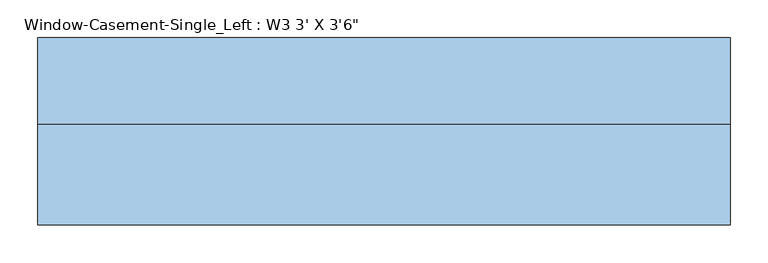
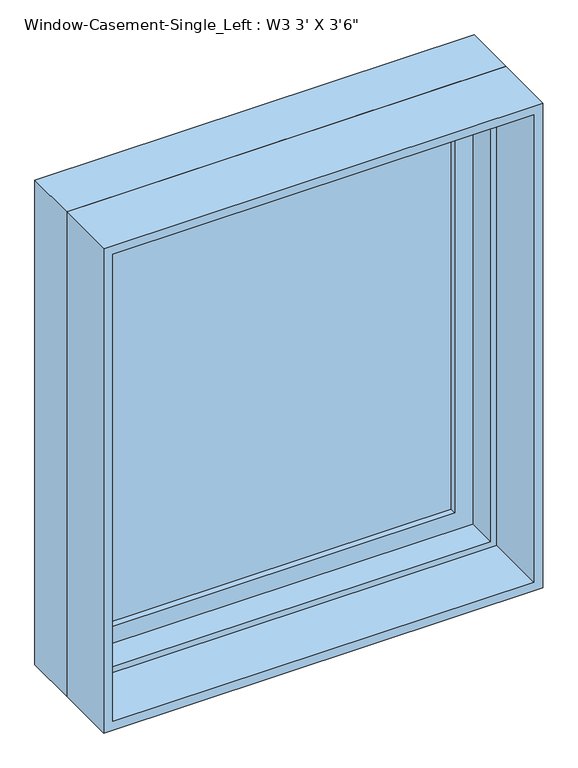
"""IFC4 building model written with IfcOpenShell, lengths in millimetres: window geometry."""

from ifc_helpers import new_model, si_unit, frame, origin, place, context, project, spatial, polyline, outline, extrude, faceted_brep, source, transform, mapped, element, save


def window_a1546d9a(model_context):
    return source(origin(), model_context, "Body", "SolidModel", [
        faceted_brep([(425.45, 82.55, 1949.45), (425.45, 19.05, 1949.45), (-425.45, 19.05, 1949.45), (-425.45, 82.55, 1949.45), (444.5, 133.35, 1968.5), (444.5, 82.55, 1968.5), (-444.5, 82.55, 1968.5), (-444.5, 133.35, 1968.5), (457.2, 19.05, 1981.2), (457.2, 133.35, 1981.2), (-457.2, 133.35, 1981.2), (-457.2, 19.05, 1981.2), (-425.45, 19.05, 946.15), (-425.45, 82.55, 946.15), (-444.5, 82.55, 927.1), (-444.5, 133.35, 927.1), (-457.2, 133.35, 914.4), (-457.2, 19.05, 914.4), (425.45, 19.05, 946.15), (425.45, 82.55, 946.15), (444.5, 82.55, 927.1), (444.5, 133.35, 927.1), (457.2, 133.35, 914.4), (457.2, 19.05, 914.4)], [[[0, 1, 2, 3]], [[4, 5, 6, 7]], [[8, 9, 10, 11]], [[3, 2, 12, 13]], [[7, 6, 14, 15]], [[11, 10, 16, 17]], [[13, 12, 18, 19]], [[15, 14, 20, 21]], [[17, 16, 22, 23]], [[11, 17, 23, 8], [1, 18, 12, 2]], [[19, 18, 1, 0]], [[5, 20, 14, 6], [3, 13, 19, 0]], [[21, 20, 5, 4]], [[23, 22, 9, 8]], [[9, 22, 16, 10], [7, 15, 21, 4]]]),
        extrude(outline(polyline([(1981.2, -457.2), (914.4, -457.2), (914.4, 457.2), (1981.2, 457.2), (1981.2, -457.2)]), holes=[polyline([(1962.15, 438.15), (933.45, 438.15), (933.45, -438.15), (1962.15, -438.15), (1962.15, 438.15)])]), frame((0.0, -114.3, 0.0), z_axis=(0.0, 1.0, 0.0), x_axis=(0.0, 0.0, 1.0)), (0.0, 0.0, 1.0), 133.35),
        extrude(outline(polyline([(1968.5, -444.5), (927.1, -444.5), (927.1, 444.5), (1968.5, 444.5), (1968.5, -444.5)]), holes=[polyline([(1911.35, 387.35), (984.25, 387.35), (984.25, -387.35), (1911.35, -387.35), (1911.35, 387.35)])]), frame((0.0, 82.55, 0.0), z_axis=(0.0, 1.0, 0.0), x_axis=(0.0, 0.0, 1.0)), (0.0, 0.0, 1.0), 44.45),
        extrude(outline(polyline([(387.35, 114.3), (387.35, 107.95), (-387.35, 107.95), (-387.35, 114.3), (387.35, 114.3)])), frame((0.0, 0.0, 984.25), z_axis=(0.0, 0.0, 1.0), x_axis=(1.0, 0.0, 0.0)), (0.0, 0.0, 1.0), 927.1),
        extrude(outline(polyline([(-387.35, 95.25), (-387.35, 101.6), (387.35, 101.6), (387.35, 95.25), (-387.35, 95.25)])), frame((0.0, 0.0, 984.25), z_axis=(0.0, 0.0, 1.0), x_axis=(1.0, 0.0, 0.0)), (0.0, 0.0, 1.0), 927.1),
    ])


if __name__ == "__main__":
    model = new_model("IFC4")
    model_context = context("Model", 3, world=origin())
    ifc_project = project(units=[si_unit("LENGTHUNIT", "METRE", prefix="MILLI")], contexts=[model_context])
    site = spatial("IfcSite", under=ifc_project)
    building = spatial("IfcBuilding", under=site)
    placement = place(None, origin())
    window_shape = window_a1546d9a(model_context)
    element("IfcWindow", 1, ObjectType="Window-Casement-Single_Left : W3 3' X 3'6\"", at=placement, inside=building, context=model_context, shape_type="MappedRepresentation", body=[
        mapped(window_shape, transform((0.0, 0.0, 0.0), x_axis=(1.0, 0.0, 0.0), y_axis=(0.0, 1.0, 0.0), z_axis=(0.0, 0.0, 1.0))),
    ])
    save(model, "model.ifc")

# Revit data of these elements
# Type "Window-Casement-Single_Left : W3 3' X 3'6\""
#   Type Mark = "20"
#   Fire Rating = "0.5h"
#   Assembly Code = "B2020100"
#   Analytic Construction = "Double glazing - domestic"
#   Window Inset [instance default] = 0' - 0"
#   Wall Thickness [instance default] = 0' - 6"
#   Visual Light Transmittance = 0.81
#   Thermal Resistance (R) = 1.8146 (h·ft²·°F)/BTU
#   Solar Heat Gain Coefficient = 0.76
#   Rough Width = 3' - 0 1/2"
#   Rough Height = 3' - 6 1/2"
#   Interior Wall Closure [instance default] = 0' - 2 1/4"
#   Height = 3' - 6"
#   Heat Transfer Coefficient (U) = 0.5511 BTU/(h·ft²·°F)
#   Frame Extension [instance default] = 0' - 0 1/4"
#   Exterior Wall Closure [instance default] = 0' - 1 1/4"
#   Extension Jamb [instance default] = 0' - 2 1/4"
#   Default Sill Height = 3' - 0"
#   Width = 3' - 0"
#   Muntin Visibility = yes
#   Interior Trim Visibility [instance default] = yes
#   Exterior Trim Visibility [instance default] = yes
#   Extension Jamb Visibility [instance default] = yes
#   Muntin Pattern = Muntin Pattern_2x2 : Muntin Pattern_2x2
#   Interior Trim Material = Wood - Stained
#   Interior Trim = Trim-Window-Interior-Flat : Picture Frame
#   Interior Frame Material = Wood - Stained
#   Glass Panel Material = Glass
#   Exterior Trim Material = Clad - White
#   Exterior Trim = Trim-Window-Exterior-Flat : with Sill
#   Exterior Frame Material = Clad - White
#   Wall Closure = (empty or 0)
# Element 1 (IfcWindow, "Window-Casement-Single_Left : W3 3' X 3'6\"")
#   Wall Thickness = 0' - 9"
#   Extension Jamb = 0' - 5 1/4"
#   Materials on its faces: "Wood - Stained", "Glass", "Clad - White"
# Materials
#   "Wood - Stained": class "Wood", colour RGB 224 178 126, transparency 0, Cost = 0
#   "Glass": class "Glass", colour RGB 0 128 192, transparency 0.75, Description = "Soda Lime Glass", Cost = 0
#   "Clad - White": class "Wood", colour RGB 242 242 238, transparency 0, Cost = 0
